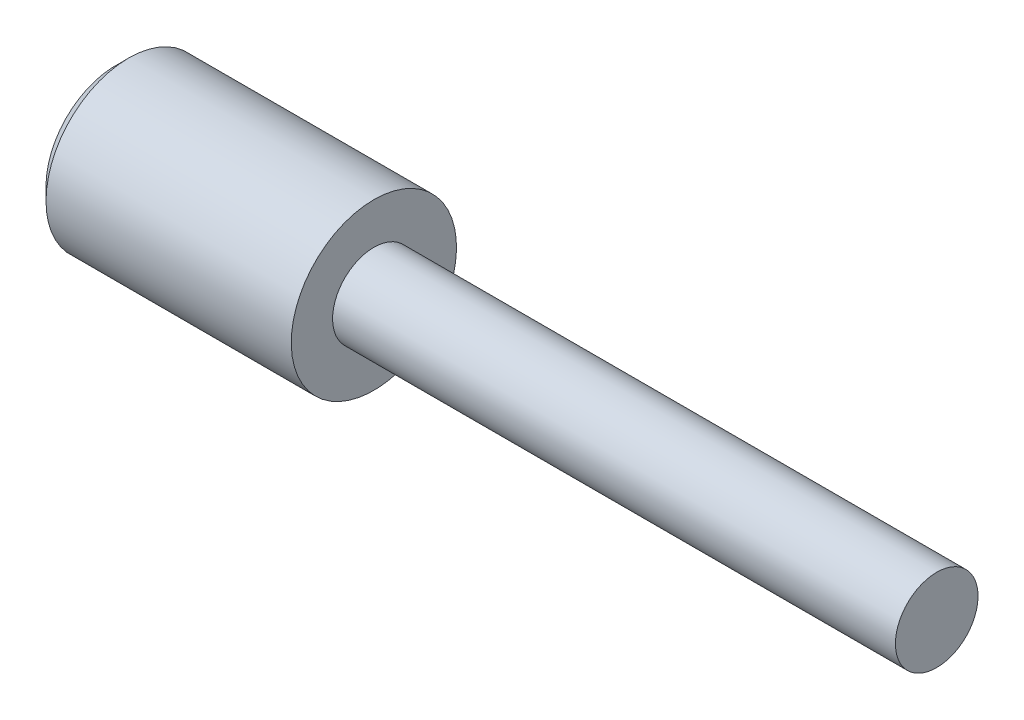
SolidWorks part; units mm, degrees
material "Plain Carbon Steel"
ref_plane "Front Plane" through (0, 0, 0) normal (0, 0, 1) x (1, 0, 0)
ref_plane "Top Plane" through (0, 0, 0) normal (0, 1, 0) x (1, 0, 0)
ref_plane "Right Plane" through (0, 0, 0) normal (1, 0, 0) x (0, 0, -1)
sketch "Shaft Profile" plane through (0, 0, 0) normal (0, 0, 1) x (1, 0, 0)
  line L0 (96.8788, 2.3205) -> (-221.1212, 2.3205)
  line L1 (-121.1212, 34.3205) -> (-221.1212, 34.3205)
  line L2 (-121.1212, 34.3205) -> (-121.1212, 18.3205)
  line L4 (-221.1212, 34.3205) -> (-221.1212, 2.3205)
  line L7 (-121.1212, 18.3205) -> (96.8788, 18.3205)
  line L11 (96.8788, 18.3205) -> (96.8788, 2.3205)
  point P0 (-171.1212, 2.3205)
  point P6 (-121.1212, 2.3205)
  dimension "D1" = 100
  dimension "D2" = 32
  dimension "218" = 218
  dimension "D3" = 16
  dimension "D4" = 50
  dimension "D5" = 221.1212
  dimension "D6" = 2.3205
revolve "Shaft Body Revolve" add sketch "Shaft Profile" angle 360 about L0
chamfer "End Chamfer 5x45°" distance 5 angle 45 1 edges at (-221.1212, 34.3205, 0)
